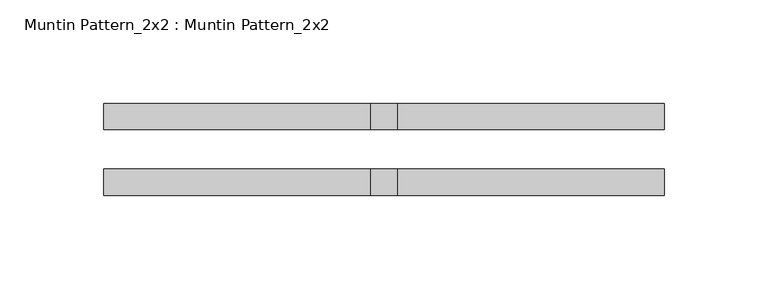
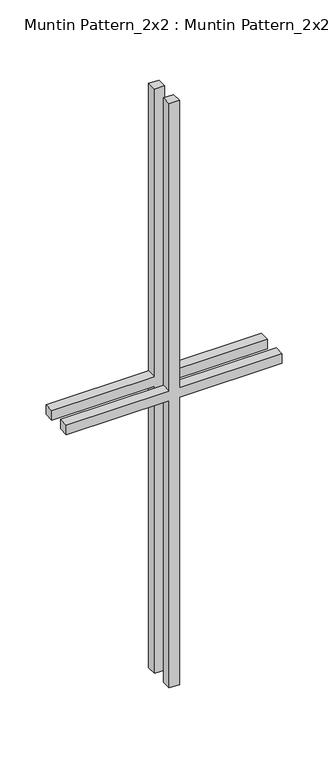
"""IFC4 building model written with IfcOpenShell, lengths in millimetres: proxy geometry, Muntin Pattern_2x2 : Muntin Pattern_2x2."""

from ifc_helpers import new_model, si_unit, frame, origin, place, context, project, spatial, polyline, outline, extrude, source, transform, mapped, element, save


def muntin_pattern_2x2_muntin_pattern_2x2_e8cdcc2d(model_context):
    return source(origin(), model_context, "Body", "SweptSolid", [
        extrude(outline(polyline([(393.7, -6.35), (393.7, -135.4666667), (381.0, -135.4666667), (381.0, -6.35), (0.0, -6.35), (0.0, 6.35), (381.0, 6.35), (381.0, 135.4666667), (393.7, 135.4666667), (393.7, 6.35), (774.7, 6.35), (774.7, -6.35), (393.7, -6.35)])), frame((0.0, -22.225, 0.0), z_axis=(0.0, 1.0, 0.0), x_axis=(0.0, 0.0, 1.0)), (0.0, 0.0, 1.0), 12.7),
        extrude(outline(polyline([(393.7, -6.35), (393.7, -135.4666667), (381.0, -135.4666667), (381.0, -6.35), (0.0, -6.35), (0.0, 6.35), (381.0, 6.35), (381.0, 135.4666667), (393.7, 135.4666667), (393.7, 6.35), (774.7, 6.35), (774.7, -6.35), (393.7, -6.35)])), frame((0.0, 9.525, 0.0), z_axis=(0.0, 1.0, 0.0), x_axis=(0.0, 0.0, 1.0)), (0.0, 0.0, 1.0), 12.7),
    ])


if __name__ == "__main__":
    model = new_model("IFC4")
    model_context = context("Model", 3, world=origin())
    ifc_project = project(units=[si_unit("LENGTHUNIT", "METRE", prefix="MILLI")], contexts=[model_context])
    site = spatial("IfcSite", under=ifc_project)
    building = spatial("IfcBuilding", under=site)
    placement = place(None, origin())
    muntin_pattern_2x2_muntin_pattern_2x2_shape = muntin_pattern_2x2_muntin_pattern_2x2_e8cdcc2d(model_context)
    element("IfcBuildingElementProxy", 1, Name="Muntin Pattern_2x2 : Muntin Pattern_2x2", ObjectType="Muntin Pattern_2x2 : Muntin Pattern_2x2", at=placement, inside=building, context=model_context, shape_type="MappedRepresentation", body=[
        mapped(muntin_pattern_2x2_muntin_pattern_2x2_shape, transform((0.0, 0.0, 0.0), x_axis=(1.0, 0.0, 0.0), y_axis=(0.0, 1.0, 0.0), z_axis=(0.0, 0.0, 1.0))),
    ])
    save(model, "model.ifc")

# Revit data of these elements
# Type "Muntin Pattern_2x2 : Muntin Pattern_2x2"
#   Width [instance default] = 4' - 0"
#   Thickness = 0' - 0 1/2"
#   Height [instance default] = 4' - 0"
#   Distance = 0' - 0 3/4"
#   Interior Material [instance default] = none
#   Exterior Material [instance default] = none
#   Default Elevation = 0
# Element 1 (IfcBuildingElementProxy, "Muntin Pattern_2x2 : Muntin Pattern_2x2")
#   Width = 0' - 10.66667"
#   Height = 2' - 6 1/2"
#   Interior Material = Wood - Stained
#   Exterior Material = Clad - White
#   Materials on its faces: "Clad - White", "Wood - Stained"
# Materials
#   "Clad - White": class "Wood", colour RGB 242 242 238, transparency 0, Cost = 0
#   "Wood - Stained": class "Wood", colour RGB 224 178 126, transparency 0, Cost = 0
